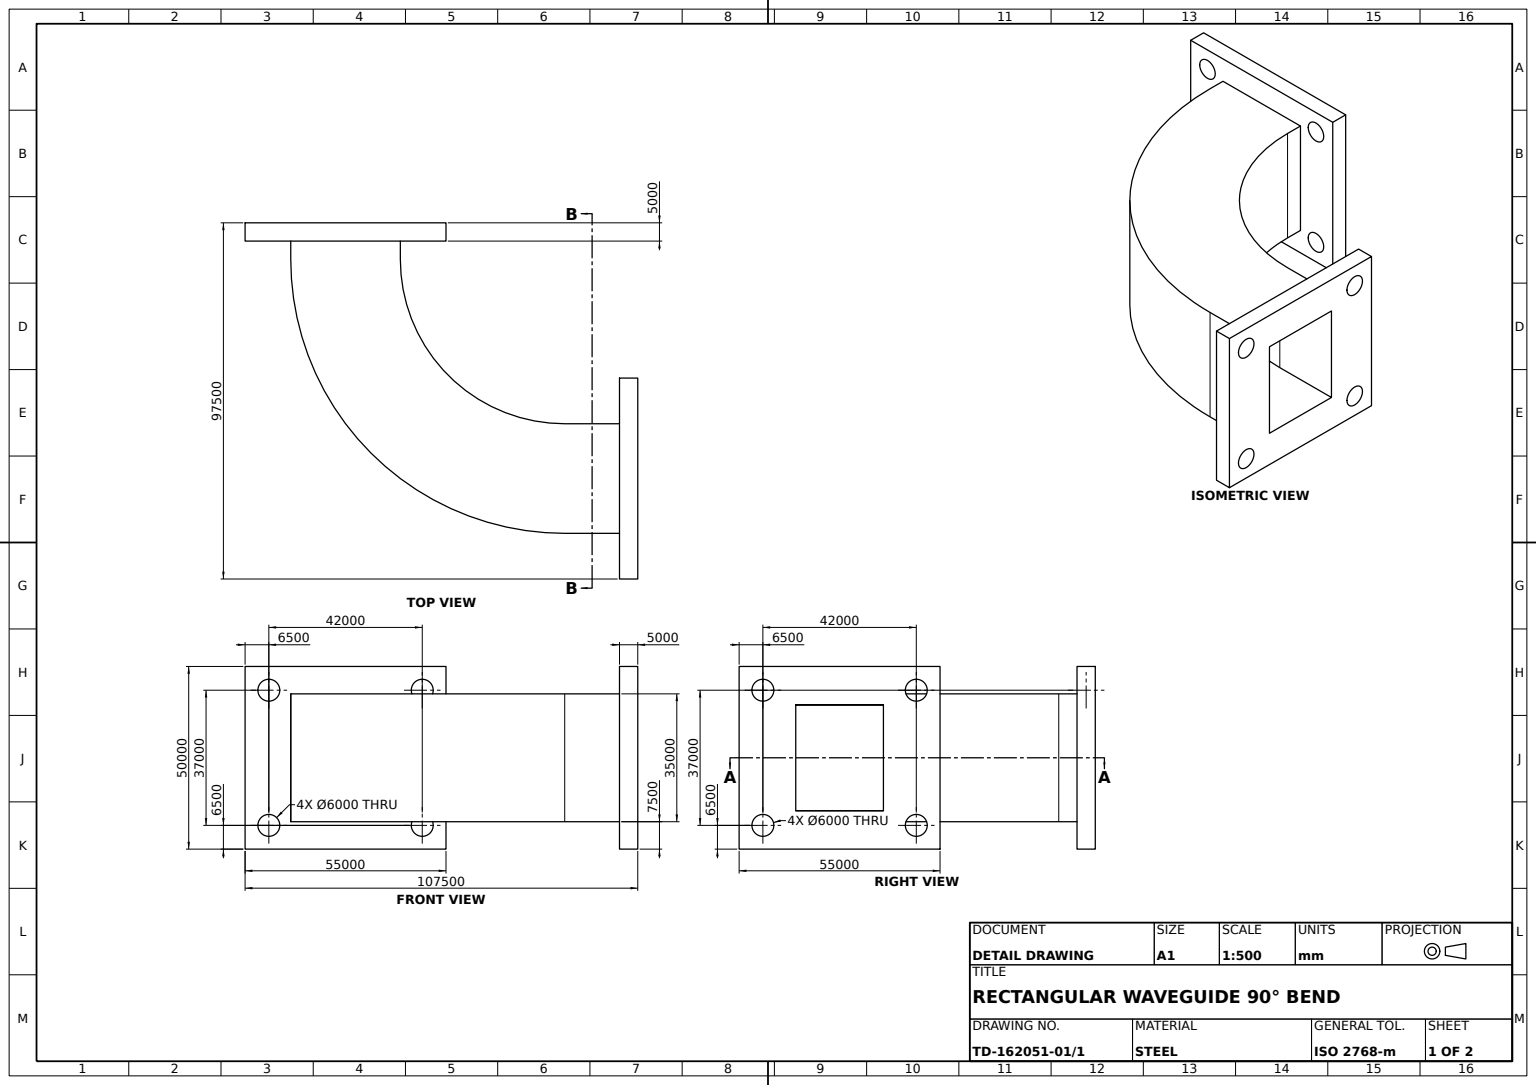
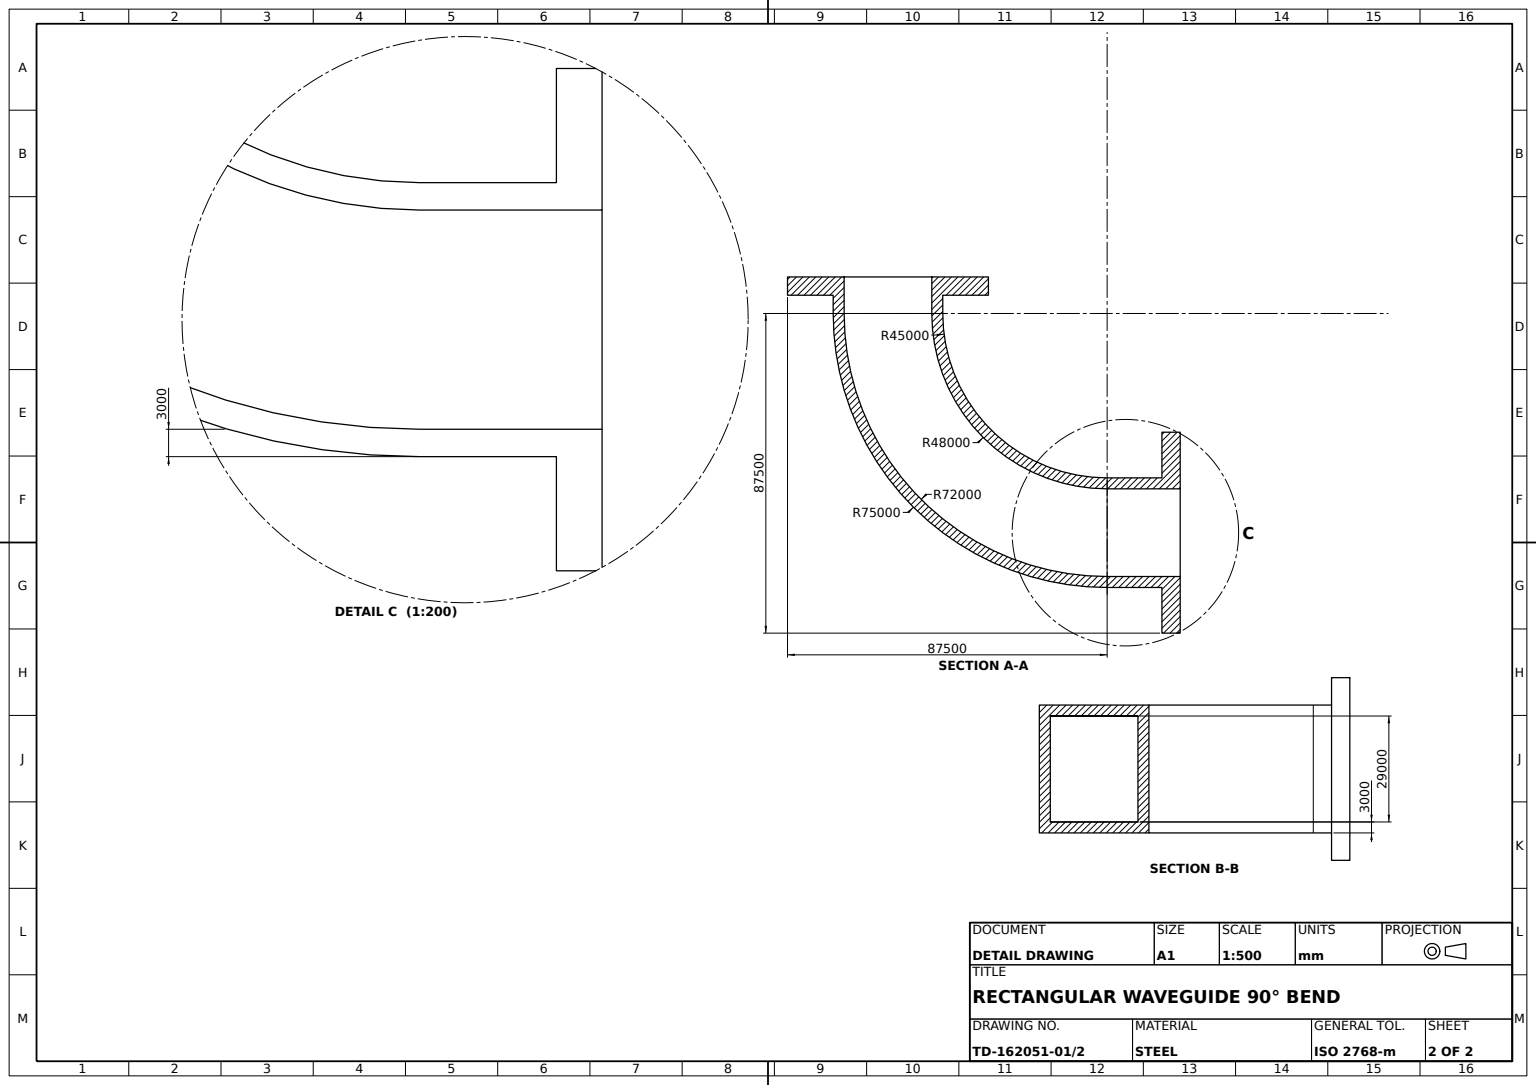
from build123d import *

# Parameters (mm, degrees)
DUCT_PROFILE_SKETCH_W        = 30000
DUCT_PROFILE_SKETCH_H        = 35000
DUCT_PROFILE_SKETCH_W_2      = 24000
DUCT_PROFILE_SKETCH_H_2      = 29000
FLANGE_A_SKETCH_W            = 55000
FLANGE_A_SKETCH_H            = 50000
FLANGE_A_SKETCH_W_2          = 24000
FLANGE_A_SKETCH_H_2          = 29000
FLANGE_A_DEPTH               = 5000
FLANGE_B_SKETCH_W            = 55000
FLANGE_B_SKETCH_H            = 50000
FLANGE_B_SKETCH_W_2          = 24000
FLANGE_B_SKETCH_H_2          = 29000
FLANGE_B_DEPTH               = 5000
FLANGE_B_BOLT_HOLES_4X_REACH = 144007.208
FLANGE_B_BOLT_HOLES_SKETCH_R = 3000
FLANGE_A_BOLT_HOLES_4X_REACH = 128575.909
FLANGE_A_BOLT_HOLES_SKETCH_R = 3000


with BuildPart() as part:
    # Duct Elbow Thin Sweep: sweep along a path in Elbow Path Sketch
    with BuildLine(Plane(origin=(0, 0, 0), x_dir=(1, 0, 0), z_dir=(0, 1, 0))) as duct_elbow_thin_sweep_path:
        Line((0, 0), (5000, 0))
        ThreePointArc((5000, 0), (47426.406871193, 17573.593128807), (65000, 60000))
        Line((65000, 60000), (65000, 75000))
    # Duct Profile Sketch → Duct Elbow Thin Sweep (sweep)
    with BuildSketch(Plane(origin=(0, 0, 0), x_dir=(0, 0, -1), z_dir=(1, 0, 0))):
        Rectangle(DUCT_PROFILE_SKETCH_W, DUCT_PROFILE_SKETCH_H)
        Rectangle(DUCT_PROFILE_SKETCH_W_2, DUCT_PROFILE_SKETCH_H_2, mode=Mode.SUBTRACT)
    sweep(path=duct_elbow_thin_sweep_path.line)

    # Flange A Sketch → Flange A (add)
    with BuildSketch(Plane.ZY):
        Rectangle(FLANGE_A_SKETCH_W, FLANGE_A_SKETCH_H)
        Rectangle(FLANGE_A_SKETCH_W_2, FLANGE_A_SKETCH_H_2, mode=Mode.SUBTRACT)
    extrude(amount=FLANGE_A_DEPTH)

    # Flange B Sketch → Flange B (add)
    with BuildSketch(Plane(origin=(0, 0, -75000), x_dir=(-1, 0, 0), z_dir=(0, 0, -1))):
        with Locations((-65000, 0)):
            Rectangle(FLANGE_B_SKETCH_W, FLANGE_B_SKETCH_H)
        with Locations((-65000, 0)):
            Rectangle(FLANGE_B_SKETCH_W_2, FLANGE_B_SKETCH_H_2, mode=Mode.SUBTRACT)
    extrude(amount=FLANGE_B_DEPTH)

    # Flange B Bolt Holes Sketch → Flange B Bolt Holes 4x (cut, up to next)
    with BuildSketch(Plane(origin=(0, 0, -80000), x_dir=(-1, 0, 0), z_dir=(0, 0, -1)), mode=Mode.PRIVATE) as flange_b_bolt_holes_4x_sk1:
        with Locations((-86000, 18500)):
            Circle(FLANGE_B_BOLT_HOLES_SKETCH_R)
    flange_b_bolt_holes_4x_tool1 = extrude(flange_b_bolt_holes_4x_sk1.sketch, amount=-FLANGE_B_BOLT_HOLES_4X_REACH, mode=Mode.PRIVATE) & part.part
    # Flange B Bolt Holes Sketch → Flange B Bolt Holes 4x (cut, up to next)
    with BuildSketch(Plane(origin=(0, 0, -80000), x_dir=(-1, 0, 0), z_dir=(0, 0, -1)), mode=Mode.PRIVATE) as flange_b_bolt_holes_4x_sk2:
        with Locations((-44000, 18500)):
            Circle(FLANGE_B_BOLT_HOLES_SKETCH_R)
    flange_b_bolt_holes_4x_tool2 = extrude(flange_b_bolt_holes_4x_sk2.sketch, amount=-FLANGE_B_BOLT_HOLES_4X_REACH, mode=Mode.PRIVATE) & part.part
    # Flange B Bolt Holes Sketch → Flange B Bolt Holes 4x (cut, up to next)
    with BuildSketch(Plane(origin=(0, 0, -80000), x_dir=(-1, 0, 0), z_dir=(0, 0, -1)), mode=Mode.PRIVATE) as flange_b_bolt_holes_4x_sk3:
        with Locations((-44000, -18500)):
            Circle(FLANGE_B_BOLT_HOLES_SKETCH_R)
    flange_b_bolt_holes_4x_tool3 = extrude(flange_b_bolt_holes_4x_sk3.sketch, amount=-FLANGE_B_BOLT_HOLES_4X_REACH, mode=Mode.PRIVATE) & part.part
    # Flange B Bolt Holes Sketch → Flange B Bolt Holes 4x (cut, up to next)
    with BuildSketch(Plane(origin=(0, 0, -80000), x_dir=(-1, 0, 0), z_dir=(0, 0, -1)), mode=Mode.PRIVATE) as flange_b_bolt_holes_4x_sk4:
        with Locations((-86000, -18500)):
            Circle(FLANGE_B_BOLT_HOLES_SKETCH_R)
    flange_b_bolt_holes_4x_tool4 = extrude(flange_b_bolt_holes_4x_sk4.sketch, amount=-FLANGE_B_BOLT_HOLES_4X_REACH, mode=Mode.PRIVATE) & part.part
    add(flange_b_bolt_holes_4x_tool1.solids().sort_by_distance((86000, 18500, -80000))[0], mode=Mode.SUBTRACT)
    add(flange_b_bolt_holes_4x_tool2.solids().sort_by_distance((44000, 18500, -80000))[0], mode=Mode.SUBTRACT)
    add(flange_b_bolt_holes_4x_tool3.solids().sort_by_distance((44000, -18500, -80000))[0], mode=Mode.SUBTRACT)
    add(flange_b_bolt_holes_4x_tool4.solids().sort_by_distance((86000, -18500, -80000))[0], mode=Mode.SUBTRACT)

    # Flange A Bolt Holes Sketch → Flange A Bolt Holes 4x (cut, up to next)
    with BuildSketch(Plane.ZY.offset(5000), mode=Mode.PRIVATE) as flange_a_bolt_holes_4x_sk1:
        with Locations((-21000, 18500)):
            Circle(FLANGE_A_BOLT_HOLES_SKETCH_R)
    flange_a_bolt_holes_4x_tool1 = extrude(flange_a_bolt_holes_4x_sk1.sketch, amount=-FLANGE_A_BOLT_HOLES_4X_REACH, mode=Mode.PRIVATE) & part.part
    # Flange A Bolt Holes Sketch → Flange A Bolt Holes 4x (cut, up to next)
    with BuildSketch(Plane.ZY.offset(5000), mode=Mode.PRIVATE) as flange_a_bolt_holes_4x_sk2:
        with Locations((21000, 18500)):
            Circle(FLANGE_A_BOLT_HOLES_SKETCH_R)
    flange_a_bolt_holes_4x_tool2 = extrude(flange_a_bolt_holes_4x_sk2.sketch, amount=-FLANGE_A_BOLT_HOLES_4X_REACH, mode=Mode.PRIVATE) & part.part
    # Flange A Bolt Holes Sketch → Flange A Bolt Holes 4x (cut, up to next)
    with BuildSketch(Plane.ZY.offset(5000), mode=Mode.PRIVATE) as flange_a_bolt_holes_4x_sk3:
        with Locations((21000, -18500)):
            Circle(FLANGE_A_BOLT_HOLES_SKETCH_R)
    flange_a_bolt_holes_4x_tool3 = extrude(flange_a_bolt_holes_4x_sk3.sketch, amount=-FLANGE_A_BOLT_HOLES_4X_REACH, mode=Mode.PRIVATE) & part.part
    # Flange A Bolt Holes Sketch → Flange A Bolt Holes 4x (cut, up to next)
    with BuildSketch(Plane.ZY.offset(5000), mode=Mode.PRIVATE) as flange_a_bolt_holes_4x_sk4:
        with Locations((-21000, -18500)):
            Circle(FLANGE_A_BOLT_HOLES_SKETCH_R)
    flange_a_bolt_holes_4x_tool4 = extrude(flange_a_bolt_holes_4x_sk4.sketch, amount=-FLANGE_A_BOLT_HOLES_4X_REACH, mode=Mode.PRIVATE) & part.part
    add(flange_a_bolt_holes_4x_tool1.solids().sort_by_distance((-5000, 18500, -21000))[0], mode=Mode.SUBTRACT)
    add(flange_a_bolt_holes_4x_tool2.solids().sort_by_distance((-5000, 18500, 21000))[0], mode=Mode.SUBTRACT)
    add(flange_a_bolt_holes_4x_tool3.solids().sort_by_distance((-5000, -18500, 21000))[0], mode=Mode.SUBTRACT)
    add(flange_a_bolt_holes_4x_tool4.solids().sort_by_distance((-5000, -18500, -21000))[0], mode=Mode.SUBTRACT)


solid = part.part
